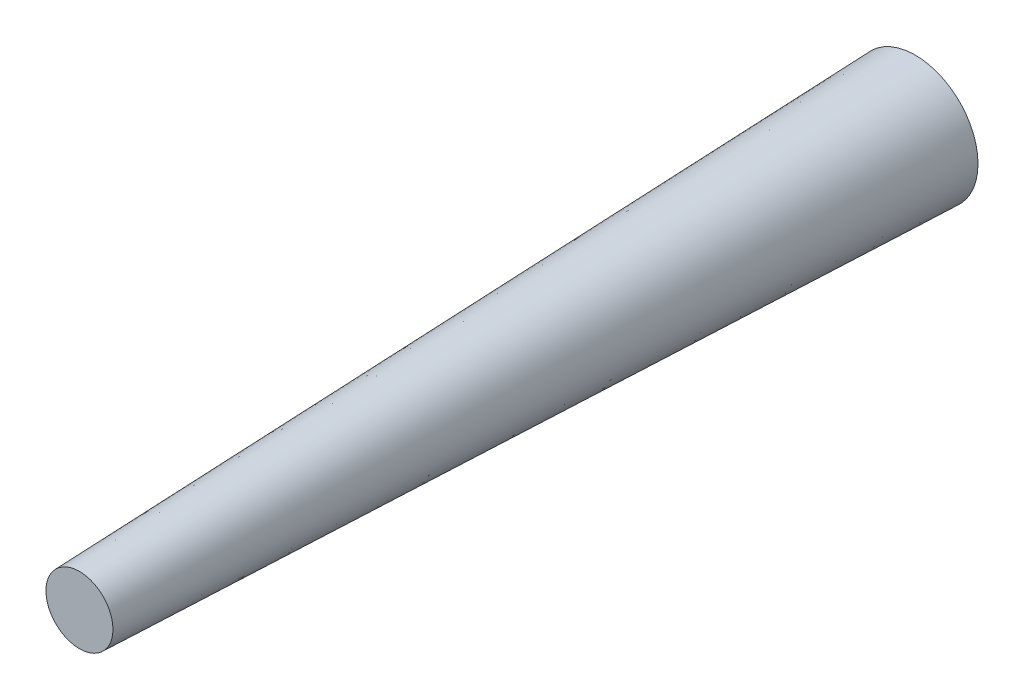
from build123d import *

# Parameters (mm, degrees)
PIN_PROFILE_6_R                   = 3
TAPER_PIN_BODY_40MM_2_DRAFT_DEPTH = 40
TAPER_PIN_BODY_40MM_2_DRAFT_TAPER = 2


with BuildPart() as part:
    # Pin Profile Ø6 → Taper Pin Body 40mm 2° Draft (new body)
    with BuildSketch(Plane.XY):
        Circle(PIN_PROFILE_6_R)
    extrude(amount=TAPER_PIN_BODY_40MM_2_DRAFT_DEPTH, taper=TAPER_PIN_BODY_40MM_2_DRAFT_TAPER)


solid = part.part
